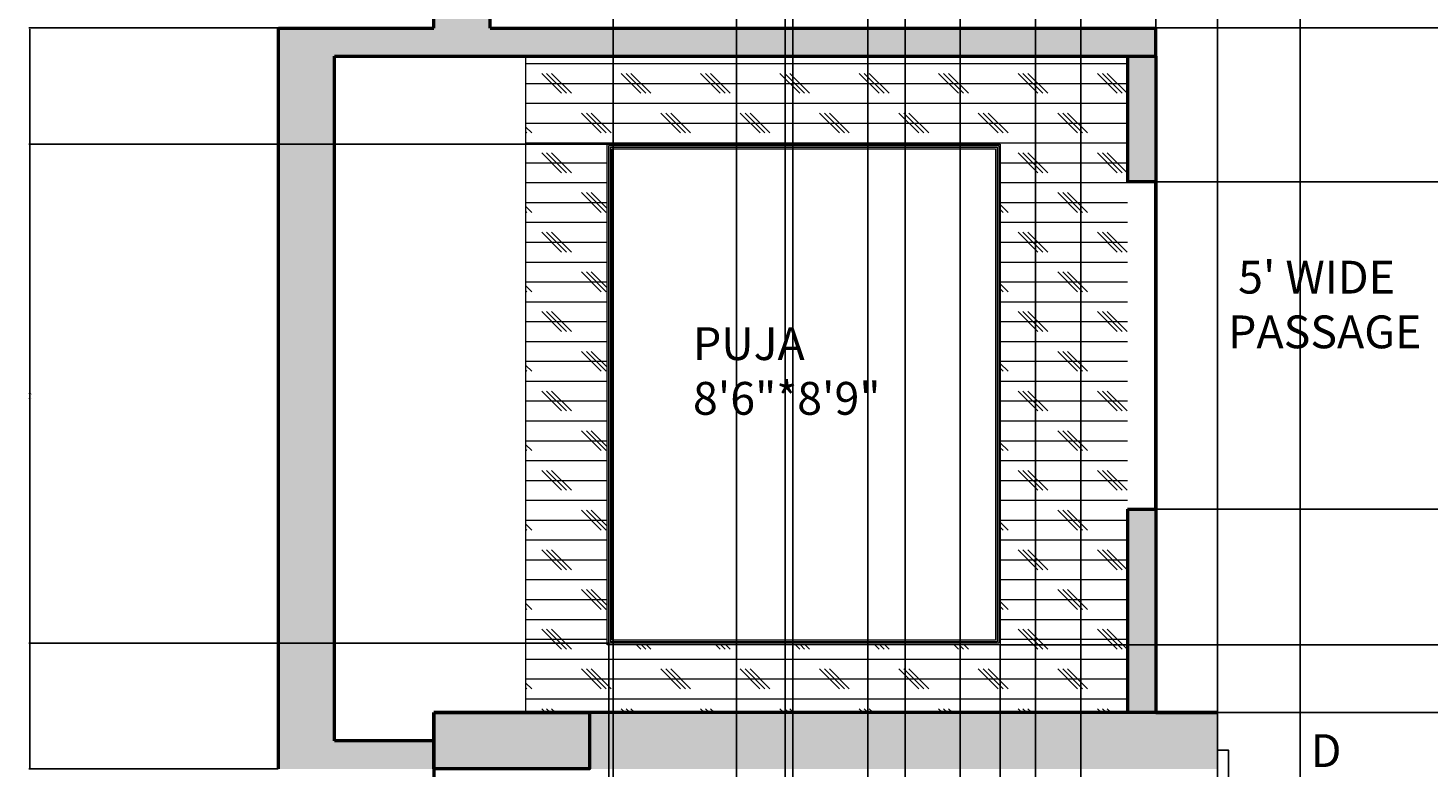
# Model space of a CAD drawing. Units: inches. Extents: x 2494 to 2908, y 1051 to 1885.
# Tile 3 of 7: x 2494 to 2718, y 1338 to 1457. Entities that reach past the tile are written whole.
import ezdxf

# ---------------------------------------------------------------- set-up
doc = ezdxf.new("R2010")
doc.units = ezdxf.units.IN
for name, color, linetype, lineweight in [('A-ANNO-DIMS', 2, 'Continuous', 18), ('A-ANNO-IDEN', 130, 'Continuous', 18), ('A-AREA-IDEN', 130, 'Continuous', 18), ('A-COLS-PATT', 200, 'Continuous', 13), ('A-FLOR-PATT', 230, 'Continuous', 13), ('A-WALL-PATT', 140, 'Continuous', 13), ('COLUMN', 200, 'Continuous', 50), ('DOOR', 50, 'Continuous', 25), ('WALL', 140, 'Continuous', 50)]:
    doc.layers.add(name, color=color, linetype=linetype, lineweight=lineweight)
doc.styles.get("Standard").update_dxf_attribs({"font": 'arial.ttf'})
doc.dimstyles.get("Standard").update_dxf_attribs({"dimtxt": 0.18, "dimasz": 0.18, "dimexe": 0.18, "dimexo": 0.0625, "dimgap": 0.09, "dimtad": 0, "dimtih": 1, "dimtoh": 1, "dimdec": 4, "dimzin": 0, "dimdsep": 46, "dimtxsty": 'Standard', "dimcen": 0.09, "dimadec": 0, "dimazin": 0, "dimtfac": 1, "dimtdec": 4, "dimtofl": 0, "dimtmove": 0, "dimatfit": 3, "dimfxl": 1, "dimtolj": 1, "dimtzin": 0, "dimarcsym": 0})

# ---------------------------------------------------------------- blocks, each defined once
blk = doc.blocks.new('*U2')
for p, q in [((0, 0), (0, -6)), ((40, 0), (40, -6))]:
    blk.add_line(p, q)
blk.add_lwpolyline([(0, 0), (0, 40), (1.75, 40), (1.75, 0)], close=True)
blk.add_arc((0, 0), 40, 0, 90)
blk = doc.blocks.new('*D28')
at = {"layer": 'A-ANNO-DIMS', "color": 0, "lineweight": -2, "transparency": 16777216}
for p, q in [((2534.34, 1456.66), (2494.47, 1456.66)), ((2494.65, 1456.48), (2494.65, 1397.59)), ((2494.65, 1338.34), (2494.65, 1397.22)), ((2534.34, 1338.16), (2494.47, 1338.16))]:
    blk.add_line(p, q, dxfattribs=at)
at = {"layer": 'A-ANNO-DIMS', "color": 0, "lineweight": 100, "transparency": 16777216}
for points in [[(2494.62, 1456.48), (2494.68, 1456.48), (2494.65, 1456.66)], [(2494.62, 1338.34), (2494.68, 1338.34), (2494.65, 1338.16)]]:
    blk.add_solid(points, dxfattribs=at)
at = {"layer": 'Defpoints', "color": 0, "lineweight": 100, "transparency": 16777216}
for p in [(2494.65, 1456.66), (2534.4, 1456.66), (2534.4, 1338.16)]:
    blk.add_point(p, dxfattribs=at)
at = {"layer": 'A-ANNO-DIMS', "color": 0, "transparency": 16777216, "insert": (2494.65, 1397.41), "char_height": 0.18, "attachment_point": 5}
blk.add_mtext('\\A1;118.5', dxfattribs=at)
blk = doc.blocks.new('*D33')
at = {"layer": 'A-ANNO-DIMS', "color": 0, "lineweight": -2, "transparency": 16777216}
for p, q in [((2697.84, 1155.22), (2697.84, 1885.09)), ((2698.02, 1884.91), (2716.38, 1884.91)), ((2735.54, 1884.91), (2717.17, 1884.91)), ((2735.72, 1155.22), (2735.72, 1885.09))]:
    blk.add_line(p, q, dxfattribs=at)
at = {"layer": 'A-ANNO-DIMS', "color": 0, "lineweight": 100, "transparency": 16777216}
for points in [[(2698.02, 1884.94), (2698.02, 1884.88), (2697.84, 1884.91)], [(2735.54, 1884.94), (2735.54, 1884.88), (2735.72, 1884.91)]]:
    blk.add_solid(points, dxfattribs=at)
at = {"layer": 'Defpoints', "color": 0, "lineweight": 100, "transparency": 16777216}
for p in [(2735.72, 1884.91), (2697.84, 1155.16), (2735.72, 1155.16)]:
    blk.add_point(p, dxfattribs=at)
at = {"layer": 'A-ANNO-DIMS', "color": 0, "transparency": 16777216, "insert": (2716.78, 1884.91), "char_height": 0.18, "attachment_point": 5}
blk.add_mtext('\\A1;37.88', dxfattribs=at)
blk = doc.blocks.new('*D34')
at = {"layer": 'A-ANNO-DIMS', "color": 0, "lineweight": -2, "transparency": 16777216}
for p, q in [((2634.69, 1155.22), (2634.69, 1885.09)), ((2634.87, 1884.91), (2665.87, 1884.91)), ((2697.66, 1884.91), (2666.66, 1884.91)), ((2697.84, 1155.22), (2697.84, 1885.09))]:
    blk.add_line(p, q, dxfattribs=at)
at = {"layer": 'A-ANNO-DIMS', "color": 0, "lineweight": 100, "transparency": 16777216}
for points in [[(2634.87, 1884.94), (2634.87, 1884.88), (2634.69, 1884.91)], [(2697.66, 1884.94), (2697.66, 1884.88), (2697.84, 1884.91)]]:
    blk.add_solid(points, dxfattribs=at)
at = {"layer": 'Defpoints', "color": 0, "lineweight": 100, "transparency": 16777216}
for p in [(2697.84, 1884.91), (2634.69, 1155.16), (2697.84, 1155.16)]:
    blk.add_point(p, dxfattribs=at)
at = {"layer": 'A-ANNO-DIMS', "color": 0, "transparency": 16777216, "insert": (2666.26, 1884.91), "char_height": 0.18, "attachment_point": 5}
blk.add_mtext('\\A1;63.15', dxfattribs=at)
blk = doc.blocks.new('*D40')
at = {"layer": 'A-ANNO-DIMS', "color": 0, "lineweight": -2, "transparency": 16777216}
for p, q in [((2615.49, 1606.59), (2615.49, 1051.41)), ((2655.49, 1606.59), (2655.49, 1051.41)), ((2615.67, 1051.59), (2635.27, 1051.59)), ((2655.31, 1051.59), (2635.71, 1051.59))]:
    blk.add_line(p, q, dxfattribs=at)
at = {"layer": 'A-ANNO-DIMS', "color": 0, "lineweight": 100, "transparency": 16777216}
for points in [[(2615.67, 1051.62), (2615.67, 1051.56), (2615.49, 1051.59)], [(2655.31, 1051.62), (2655.31, 1051.56), (2655.49, 1051.59)]]:
    blk.add_solid(points, dxfattribs=at)
at = {"layer": 'Defpoints', "color": 0, "lineweight": 100, "transparency": 16777216}
for p in [(2615.49, 1606.66), (2655.49, 1606.66), (2655.49, 1051.59)]:
    blk.add_point(p, dxfattribs=at)
at = {"layer": 'A-ANNO-DIMS', "color": 0, "transparency": 16777216, "insert": (2635.49, 1051.59), "char_height": 0.18, "attachment_point": 5}
blk.add_mtext('\\A1;40', dxfattribs=at)
blk = doc.blocks.new('*D41')
at = {"layer": 'A-ANNO-DIMS', "color": 0, "lineweight": -2, "transparency": 16777216}
for p, q in [((2684.64, 1347.22), (2684.64, 1885.09)), ((2684.82, 1884.91), (2704.42, 1884.91)), ((2724.46, 1884.91), (2704.86, 1884.91)), ((2724.64, 1347.22), (2724.64, 1885.09))]:
    blk.add_line(p, q, dxfattribs=at)
at = {"layer": 'A-ANNO-DIMS', "color": 0, "lineweight": 100, "transparency": 16777216}
for points in [[(2684.82, 1884.94), (2684.82, 1884.88), (2684.64, 1884.91)], [(2724.46, 1884.94), (2724.46, 1884.88), (2724.64, 1884.91)]]:
    blk.add_solid(points, dxfattribs=at)
at = {"layer": 'Defpoints', "color": 0, "lineweight": 100, "transparency": 16777216}
for p in [(2724.64, 1884.91), (2684.64, 1347.16), (2724.64, 1347.16)]:
    blk.add_point(p, dxfattribs=at)
at = {"layer": 'A-ANNO-DIMS', "color": 0, "transparency": 16777216, "insert": (2704.64, 1884.91), "char_height": 0.18, "attachment_point": 5}
blk.add_mtext('\\A1;40', dxfattribs=at)
blk = doc.blocks.new('*D42')
at = {"layer": 'A-ANNO-DIMS', "color": 0, "lineweight": -2, "transparency": 16777216}
for p, q in [((2674.75, 1347.22), (2674.75, 1885.09)), ((2674.93, 1884.91), (2679.3, 1884.91)), ((2684.46, 1884.91), (2680.09, 1884.91)), ((2684.64, 1347.22), (2684.64, 1885.09))]:
    blk.add_line(p, q, dxfattribs=at)
at = {"layer": 'A-ANNO-DIMS', "color": 0, "lineweight": 100, "transparency": 16777216}
for points in [[(2674.93, 1884.94), (2674.93, 1884.88), (2674.75, 1884.91)], [(2684.46, 1884.94), (2684.46, 1884.88), (2684.64, 1884.91)]]:
    blk.add_solid(points, dxfattribs=at)
at = {"layer": 'Defpoints', "color": 0, "lineweight": 100, "transparency": 16777216}
for p in [(2684.64, 1884.91), (2674.75, 1347.16), (2684.64, 1347.16)]:
    blk.add_point(p, dxfattribs=at)
at = {"layer": 'A-ANNO-DIMS', "color": 0, "transparency": 16777216, "insert": (2679.7, 1884.91), "char_height": 0.18, "attachment_point": 5}
blk.add_mtext('\\A1;9.889', dxfattribs=at)
blk = doc.blocks.new('*D46')
at = {"layer": 'A-ANNO-DIMS', "color": 0, "lineweight": -2, "transparency": 16777216}
for p, q in [((2674.81, 1432.05), (2908.18, 1432.05)), ((2908, 1431.87), (2908, 1406.05)), ((2908, 1379.87), (2908, 1405.69)), ((2674.81, 1379.69), (2908.18, 1379.69))]:
    blk.add_line(p, q, dxfattribs=at)
at = {"layer": 'A-ANNO-DIMS', "color": 0, "lineweight": 100, "transparency": 16777216}
for points in [[(2907.97, 1431.87), (2908.03, 1431.87), (2908, 1432.05)], [(2907.97, 1379.87), (2908.03, 1379.87), (2908, 1379.69)]]:
    blk.add_solid(points, dxfattribs=at)
at = {"layer": 'Defpoints', "color": 0, "lineweight": 100, "transparency": 16777216}
for p in [(2674.75, 1432.05), (2908, 1432.05), (2674.75, 1379.69)]:
    blk.add_point(p, dxfattribs=at)
at = {"layer": 'A-ANNO-DIMS', "color": 0, "transparency": 16777216, "insert": (2908, 1405.87), "char_height": 0.18, "attachment_point": 5}
blk.add_mtext('\\A1;52.36', dxfattribs=at)
blk = doc.blocks.new('*D47')
at = {"layer": 'A-ANNO-DIMS', "color": 0, "lineweight": -2, "transparency": 16777216}
for p, q in [((2674.81, 1456.66), (2908.18, 1456.66)), ((2908, 1456.48), (2908, 1444.53)), ((2908, 1432.23), (2908, 1444.17)), ((2674.81, 1432.05), (2908.18, 1432.05))]:
    blk.add_line(p, q, dxfattribs=at)
at = {"layer": 'A-ANNO-DIMS', "color": 0, "lineweight": 100, "transparency": 16777216}
for points in [[(2907.97, 1456.48), (2908.03, 1456.48), (2908, 1456.66)], [(2907.97, 1432.23), (2908.03, 1432.23), (2908, 1432.05)]]:
    blk.add_solid(points, dxfattribs=at)
at = {"layer": 'Defpoints', "color": 0, "lineweight": 100, "transparency": 16777216}
for p in [(2674.75, 1456.66), (2908, 1456.66), (2674.75, 1432.05)]:
    blk.add_point(p, dxfattribs=at)
at = {"layer": 'A-ANNO-DIMS', "color": 0, "transparency": 16777216, "insert": (2908, 1444.35), "char_height": 0.18, "attachment_point": 5}
blk.add_mtext('\\A1;24.606', dxfattribs=at)
blk = doc.blocks.new('*D49')
at = {"layer": 'A-ANNO-DIMS', "color": 0, "lineweight": -2, "transparency": 16777216}
for p, q in [((2587.26, 1358.2), (2587.26, 1051.41)), ((2649.88, 1357.95), (2649.88, 1051.41)), ((2587.44, 1051.59), (2618.17, 1051.59)), ((2649.7, 1051.59), (2618.96, 1051.59))]:
    blk.add_line(p, q, dxfattribs=at)
at = {"layer": 'A-ANNO-DIMS', "color": 0, "lineweight": 100, "transparency": 16777216}
for points in [[(2587.44, 1051.62), (2587.44, 1051.56), (2587.26, 1051.59)], [(2649.7, 1051.62), (2649.7, 1051.56), (2649.88, 1051.59)]]:
    blk.add_solid(points, dxfattribs=at)
at = {"layer": 'Defpoints', "color": 0, "lineweight": 100, "transparency": 16777216}
for p in [(2587.26, 1358.26), (2649.88, 1358.01), (2649.88, 1051.59)]:
    blk.add_point(p, dxfattribs=at)
at = {"layer": 'A-ANNO-DIMS', "color": 0, "transparency": 16777216, "insert": (2618.57, 1051.59), "char_height": 0.18, "attachment_point": 5}
blk.add_mtext('\\A1;62.62', dxfattribs=at)
blk = doc.blocks.new('*D50')
at = {"layer": 'A-ANNO-DIMS', "color": 0, "lineweight": -2, "transparency": 16777216}
for p, q in [((2586.95, 1438.09), (2494.47, 1438.09)), ((2494.65, 1437.91), (2494.65, 1398.36)), ((2494.65, 1358.44), (2494.65, 1397.99)), ((2587.2, 1358.26), (2494.47, 1358.26))]:
    blk.add_line(p, q, dxfattribs=at)
at = {"layer": 'A-ANNO-DIMS', "color": 0, "lineweight": 100, "transparency": 16777216}
for points in [[(2494.62, 1437.91), (2494.68, 1437.91), (2494.65, 1438.09)], [(2494.62, 1358.44), (2494.68, 1358.44), (2494.65, 1358.26)]]:
    blk.add_solid(points, dxfattribs=at)
at = {"layer": 'Defpoints', "color": 0, "lineweight": 100, "transparency": 16777216}
for p in [(2494.65, 1438.09), (2587.01, 1438.09), (2587.26, 1358.26)]:
    blk.add_point(p, dxfattribs=at)
at = {"layer": 'A-ANNO-DIMS', "color": 0, "transparency": 16777216, "insert": (2494.65, 1398.17), "char_height": 0.18, "attachment_point": 5}
blk.add_mtext('\\A1;79.83', dxfattribs=at)
blk = doc.blocks.new('*D51')
at = {"layer": 'A-ANNO-DIMS', "color": 0, "lineweight": -2, "transparency": 16777216}
for p, q in [((2587.26, 1358.2), (2587.26, 1051.41)), ((2559.25, 1347.09), (2559.25, 1051.41)), ((2559.43, 1051.59), (2572.88, 1051.59)), ((2587.08, 1051.59), (2573.63, 1051.59))]:
    blk.add_line(p, q, dxfattribs=at)
at = {"layer": 'A-ANNO-DIMS', "color": 0, "lineweight": 100, "transparency": 16777216}
for points in [[(2559.43, 1051.62), (2559.43, 1051.56), (2559.25, 1051.59)], [(2587.08, 1051.62), (2587.08, 1051.56), (2587.26, 1051.59)]]:
    blk.add_solid(points, dxfattribs=at)
at = {"layer": 'Defpoints', "color": 0, "lineweight": 100, "transparency": 16777216}
for p in [(2587.26, 1358.26), (2559.25, 1347.16), (2559.25, 1051.59)]:
    blk.add_point(p, dxfattribs=at)
at = {"layer": 'A-ANNO-DIMS', "color": 0, "transparency": 16777216, "insert": (2573.26, 1051.59), "char_height": 0.18, "attachment_point": 5}
blk.add_mtext('\\A1;28.01', dxfattribs=at)
blk = doc.blocks.new('*D52')
at = {"layer": 'A-ANNO-DIMS', "color": 0, "lineweight": -2, "transparency": 16777216}
for p, q in [((2649.94, 1358.01), (2908.18, 1358.01)), ((2908, 1357.83), (2908, 1352.76)), ((2908, 1347.34), (2908, 1352.4)), ((2670.31, 1347.16), (2908.18, 1347.16))]:
    blk.add_line(p, q, dxfattribs=at)
at = {"layer": 'A-ANNO-DIMS', "color": 0, "lineweight": 100, "transparency": 16777216}
for points in [[(2907.97, 1357.83), (2908.03, 1357.83), (2908, 1358.01)], [(2907.97, 1347.34), (2908.03, 1347.34), (2908, 1347.16)]]:
    blk.add_solid(points, dxfattribs=at)
at = {"layer": 'Defpoints', "color": 0, "lineweight": 100, "transparency": 16777216}
for p in [(2649.88, 1358.01), (2908, 1358.01), (2670.25, 1347.16)]:
    blk.add_point(p, dxfattribs=at)
at = {"layer": 'A-ANNO-DIMS', "color": 0, "transparency": 16777216, "insert": (2908, 1352.58), "char_height": 0.18, "attachment_point": 5}
blk.add_mtext('\\A1;10.852', dxfattribs=at)
blk = doc.blocks.new('*D60')
at = {"layer": 'A-ANNO-DIMS', "color": 0, "lineweight": -2, "transparency": 16777216}
for p, q in [((2587.96, 1514.09), (2587.96, 1051.41)), ((2607.71, 1514.09), (2607.71, 1051.41)), ((2588.14, 1051.59), (2597.45, 1051.59)), ((2607.53, 1051.59), (2598.22, 1051.59))]:
    blk.add_line(p, q, dxfattribs=at)
at = {"layer": 'A-ANNO-DIMS', "color": 0, "lineweight": 100, "transparency": 16777216}
for points in [[(2588.14, 1051.62), (2588.14, 1051.56), (2587.96, 1051.59)], [(2607.53, 1051.62), (2607.53, 1051.56), (2607.71, 1051.59)]]:
    blk.add_solid(points, dxfattribs=at)
at = {"layer": 'Defpoints', "color": 0, "lineweight": 100, "transparency": 16777216}
for p in [(2587.96, 1514.15), (2607.71, 1514.15), (2607.71, 1051.59)]:
    blk.add_point(p, dxfattribs=at)
at = {"layer": 'A-ANNO-DIMS', "color": 0, "transparency": 16777216, "insert": (2597.83, 1051.59), "char_height": 0.18, "attachment_point": 5}
blk.add_mtext('\\A1;19.76', dxfattribs=at)
blk = doc.blocks.new('*D62')
at = {"layer": 'A-ANNO-DIMS', "color": 0, "lineweight": -2, "transparency": 16777216}
for p, q in [((2616.72, 1527.95), (2616.72, 1051.41)), ((2628.68, 1527.95), (2628.68, 1051.41)), ((2616.9, 1051.59), (2622.25, 1051.59)), ((2628.5, 1051.59), (2623.16, 1051.59))]:
    blk.add_line(p, q, dxfattribs=at)
at = {"layer": 'A-ANNO-DIMS', "color": 0, "lineweight": 100, "transparency": 16777216}
for points in [[(2616.9, 1051.62), (2616.9, 1051.56), (2616.72, 1051.59)], [(2628.5, 1051.62), (2628.5, 1051.56), (2628.68, 1051.59)]]:
    blk.add_solid(points, dxfattribs=at)
at = {"layer": 'Defpoints', "color": 0, "lineweight": 100, "transparency": 16777216}
for p in [(2616.72, 1528.01), (2628.68, 1528.01), (2628.68, 1051.59)]:
    blk.add_point(p, dxfattribs=at)
at = {"layer": 'A-ANNO-DIMS', "color": 0, "transparency": 16777216, "insert": (2622.7, 1051.59), "char_height": 0.18, "attachment_point": 5}
blk.add_mtext('\\A1;11.963', dxfattribs=at)
blk = doc.blocks.new('*D65')
at = {"layer": 'A-ANNO-DIMS', "color": 0, "lineweight": -2, "transparency": 16777216}
for p, q in [((2662.76, 1694.66), (2662.76, 1051.41)), ((2643.46, 1680.73), (2643.46, 1051.41)), ((2643.64, 1051.59), (2652.66, 1051.59)), ((2662.58, 1051.59), (2653.57, 1051.59))]:
    blk.add_line(p, q, dxfattribs=at)
at = {"layer": 'A-ANNO-DIMS', "color": 0, "lineweight": 100, "transparency": 16777216}
for points in [[(2643.64, 1051.62), (2643.64, 1051.56), (2643.46, 1051.59)], [(2662.58, 1051.62), (2662.58, 1051.56), (2662.76, 1051.59)]]:
    blk.add_solid(points, dxfattribs=at)
at = {"layer": 'Defpoints', "color": 0, "lineweight": 100, "transparency": 16777216}
for p in [(2662.76, 1694.72), (2643.46, 1680.79), (2662.76, 1051.59)]:
    blk.add_point(p, dxfattribs=at)
at = {"layer": 'A-ANNO-DIMS', "color": 0, "transparency": 16777216, "insert": (2653.11, 1051.59), "char_height": 0.18, "attachment_point": 5}
blk.add_mtext('\\A1;19.305', dxfattribs=at)

msp = doc.modelspace()

# ---------------------------------------------------------------- hatches: boundary and pattern name
at = {"layer": 'A-COLS-PATT'}
h = msp.add_hatch(color=256, dxfattribs=at)
h.dxf.hatch_style = 1
h.paths.add_polyline_path([(2584.1612, 1845.1561), (2559.2517, 1845.1561), (2559.2517, 1836.1561), (2584.1612, 1836.1561)])
h.paths.add_polyline_path([(2720.7462, 1845.1561), (2695.8368, 1845.1561), (2695.8368, 1836.1561), (2720.7462, 1836.1561)])
h.paths.add_polyline_path([(2868.2517, 1845.1561), (2843.3423, 1845.1561), (2843.3423, 1836.1561), (2868.2517, 1836.1561)])
h.paths.add_polyline_path([(2568.2517, 1728.1561), (2559.2517, 1728.1561), (2559.2517, 1703.2467), (2568.2517, 1703.2467)])
h.paths.add_polyline_path([(2568.2517, 1564.0885), (2559.2517, 1564.0885), (2559.2517, 1539.1791), (2568.2517, 1539.1791)])
h.paths.add_polyline_path([(2868.2517, 1554.4528), (2859.2517, 1554.4528), (2859.2517, 1529.5434), (2868.2517, 1529.5434)])
h.paths.add_polyline_path([(2806.0841, 1611.1561), (2781.1746, 1611.1561), (2781.1746, 1602.1561), (2806.0841, 1602.1561)])
h.paths.add_polyline_path([(2868.0971, 1611.1561), (2843.1877, 1611.1561), (2843.1877, 1602.1561), (2868.0971, 1602.1561)])
h.paths.add_polyline_path([(2584.1612, 1347.1561), (2559.2517, 1347.1561), (2559.2517, 1338.1561), (2584.1612, 1338.1561)])
h.paths.add_polyline_path([(2868.2517, 1347.1561), (2843.3423, 1347.1561), (2843.3423, 1338.1561), (2868.2517, 1338.1561)])
h.paths.add_polyline_path([(2568.2517, 1180.0656), (2559.2517, 1180.0656), (2559.2517, 1155.1561), (2568.2517, 1155.1561)])
h.paths.add_polyline_path([(2584.1612, 1155.1561), (2559.2517, 1155.1561), (2559.2517, 1146.1561), (2584.1612, 1146.1561)])
h.paths.add_polyline_path([(2868.2517, 1155.1561), (2843.3423, 1155.1561), (2843.3423, 1146.1561), (2868.2517, 1146.1561)])
h.paths.add_polyline_path([(2868.2517, 1180.0656), (2859.2517, 1180.0656), (2859.2517, 1155.1561), (2868.2517, 1155.1561)])
at = {"layer": 'A-FLOR-PATT'}
h = msp.add_hatch(dxfattribs=at)
h.set_pattern_fill('CORK', color=256)
h.set_pattern_definition([(0, (0, 0), (0, 3.175), []), (135, (1.5875, -1.5875), (-6.350003, -6.350003), [4.49013, -4.49013]), (135, (2.381, -1.5875), (-6.350003, -6.350003), [4.49013, -4.49013]), (135, (3.175, -1.5875), (-6.350003, -6.350003), [4.49013, -4.49013])])
h.paths.add_polyline_path([(2670.2517, 1452.1561), (2574.0043, 1452.1561), (2574.0043, 1347.1561), (2584.1612, 1347.1561), (2670.2517, 1347.1561)])
h.paths.add_polyline_path([(2649.877, 1438.0892), (2649.877, 1358.0085), (2587.0092, 1358.0085), (2587.0092, 1438.0892)], flags=16)
h.paths.add_polyline_path([(2649.627, 1437.8392), (2649.627, 1358.2585), (2587.2592, 1358.2585), (2587.2592, 1437.8392)], flags=0)
h.paths.add_polyline_path([(2649.377, 1437.5892), (2649.377, 1358.5085), (2587.5092, 1358.5085), (2587.5092, 1437.5892)], flags=0)
h.paths.add_polyline_path([(2649.127, 1437.3392), (2649.127, 1358.7585), (2587.7592, 1358.7585), (2587.7592, 1437.3392)], flags=0)
h.paths.add_polyline_path([(2598.8437, 1391.9158), (2628.9044, 1391.9158), (2628.9044, 1411.4992), (2598.8437, 1411.4992)], flags=8)
at = {"layer": 'A-WALL-PATT'}
h = msp.add_hatch(color=256, dxfattribs=at)
h.dxf.hatch_style = 1
h.paths.add_polyline_path([(2805.2517, 1547.9123), (2796.2517, 1547.9123), (2796.2517, 1530.1561), (2859.2517, 1530.1561), (2859.2517, 1539.1561), (2805.2517, 1539.1561)])
h.paths.add_polyline_path([(2568.2517, 1606.6561), (2615.4916, 1606.6561), (2615.4916, 1611.1561), (2559.2517, 1611.1561), (2559.2517, 1564.0885), (2568.2517, 1564.0885)])
h.paths.add_polyline_path([(2568.2517, 1539.1791), (2559.2517, 1539.1791), (2559.2517, 1456.6561), (2534.4016, 1456.6561), (2534.4016, 1338.1561), (2559.2517, 1338.1561), (2559.2517, 1342.6561), (2543.4016, 1342.6561), (2543.4016, 1452.1561), (2559.2517, 1452.1561), (2568.2517, 1452.1561), (2674.7517, 1452.1561), (2674.7517, 1456.6561), (2568.2517, 1456.6561)])
h.paths.add_polyline_path([(2684.6403, 1347.1561), (2674.7517, 1347.1561), (2584.1612, 1347.1561), (2584.1612, 1338.1561), (2684.6403, 1338.1561), (2684.6403, 1341.1561)])
h.paths.add_polyline_path([(2843.3423, 1347.1561), (2832.3482, 1347.1561), (2832.3482, 1338.1485), (2843.3423, 1338.1485)])
h.paths.add_polyline_path([(2634.6908, 1155.1561), (2584.1612, 1155.1561), (2584.1612, 1146.1561), (2634.6908, 1146.1561)])
h.paths.add_polyline_path([(2783.7833, 1155.1561), (2772.2517, 1155.1561), (2772.2517, 1146.1561), (2783.7833, 1146.1561)])
h.paths.add_polyline_path([(2843.3423, 1155.1561), (2819.0012, 1155.1561), (2811.9091, 1155.1561), (2811.9091, 1146.1561), (2843.3423, 1146.1561)])
h.paths.add_polyline_path([(2868.2517, 1243.6561), (2859.2517, 1243.6561), (2859.2517, 1239.1561), (2859.2517, 1180.0656), (2868.2517, 1180.0656)])
h = msp.add_hatch(color=256, dxfattribs=at)
h.dxf.hatch_style = 1
h.paths.add_polyline_path([(2674.7517, 1379.6865), (2670.2517, 1379.6865), (2670.2517, 1347.1561), (2674.7517, 1347.1561)])
h.paths.add_polyline_path([(2674.7517, 1452.1561), (2670.2517, 1452.1561), (2670.2517, 1432.0498), (2674.7517, 1432.0498)])

# ---------------------------------------------------------------- linework, layer by layer
at = {"layer": 'A-FLOR-PATT'}
msp.add_line((2574.0043, 1347.1561), (2574.0043, 1452.1561), dxfattribs=at)
for points in [[(2587.0092, 1438.0892), (2649.877, 1438.0892), (2649.877, 1358.0085), (2587.0092, 1358.0085)], [(2587.2592, 1437.8392), (2649.627, 1437.8392), (2649.627, 1358.2585), (2587.2592, 1358.2585)], [(2587.5092, 1437.5892), (2649.377, 1437.5892), (2649.377, 1358.5085), (2587.5092, 1358.5085)], [(2587.7592, 1437.3392), (2649.127, 1437.3392), (2649.127, 1358.7585), (2587.7592, 1358.7585)]]:
    msp.add_lwpolyline(points, close=True, dxfattribs=at)
at = {"layer": 'COLUMN'}
msp.add_lwpolyline([(2559.2517, 1347.1561), (2584.1612, 1347.1561), (2584.1612, 1338.1561), (2559.2517, 1338.1561)], close=True, dxfattribs=at)
at = {"layer": 'WALL'}
for p, q in [((2559.2517, 1456.6561), (2559.2517, 1611.1561)), ((2568.2517, 1456.6561), (2568.2517, 1606.6561)), ((2534.4016, 1338.1561), (2534.4016, 1456.6561)), ((2534.4016, 1456.6561), (2559.2517, 1456.6561)), ((2568.2517, 1456.6561), (2674.7517, 1456.6561)), ((2568.2517, 1456.6561), (2674.7517, 1456.6561)), ((2674.7517, 1452.1561), (2674.7517, 1456.6561)), ((2543.4016, 1342.6561), (2543.4016, 1452.1561)), ((2543.4016, 1452.1561), (2559.2517, 1452.1561)), ((2559.2517, 1452.1561), (2568.2517, 1452.1561)), ((2568.2517, 1452.1561), (2670.2517, 1452.1561)), ((2568.2517, 1452.1561), (2674.7517, 1452.1561)), ((2670.2517, 1452.1561), (2670.2517, 1432.0498)), ((2674.7517, 1452.1561), (2674.7517, 1347.1561)), ((2670.2517, 1379.6865), (2670.2517, 1347.1561)), ((2559.2517, 1347.1561), (2559.2517, 1146.1561)), ((2684.6403, 1347.1561), (2559.2517, 1347.1561)), ((2674.7517, 1347.1561), (2684.6403, 1347.1561)), ((2559.2517, 1342.6561), (2543.4016, 1342.6561))]:
    msp.add_line(p, q, dxfattribs=at)
msp.add_lwpolyline([(2670.2517, 1379.6865), (2674.7517, 1379.6865), (2674.7517, 1432.0498), (2670.2517, 1432.0498)], dxfattribs=at)

# ---------------------------------------------------------------- block references
at = {"layer": 'DOOR', "xscale": -1, "rotation": 180}
msp.add_blockref('*U2', (2684.6403, 1341.1561), dxfattribs=at)

# ---------------------------------------------------------------- texts
at = {"layer": 'A-ANNO-IDEN', "insert": (2699.5394, 1343.7052), "char_height": 5.2482, "attachment_point": 1}
msp.add_mtext_dynamic_manual_height_columns('D', width=250.978097, gutter_width=26.2409, heights=[0], dxfattribs=at)
at = {"layer": 'A-AREA-IDEN', "char_height": 5.24818, "attachment_point": 1}
for s, insert in [(" 5' WIDE\\PPASSAGE", (2686.3269, 1419.4317)), ('PUJA\\P8\'6"*8\'9"', (2600.7214, 1408.7981))]:
    msp.add_mtext_dynamic_manual_height_columns(s, width=250.978097, gutter_width=26.2409, heights=[0], dxfattribs=dict(at, insert=insert))

# ---------------------------------------------------------------- dimensions: what is measured, and where the dimension line sits
at = {"layer": 'A-ANNO-DIMS'}
for base, p1, p2, override, picture, middle in [((2697.838, 1884.9061), (2634.6908, 1155.1561), (2697.838, 1155.1561), {"dimdec": 2, "dimlfac": 1, "dimrnd": 0, "dimzin": 0, "dimdsep": 46, "dimlunit": 2}, '*D34', (2666.2644, 1884.9061)), ((2684.6403, 1884.9061), (2674.7517, 1347.1561), (2684.6403, 1347.1561), {"dimdec": 3, "dimlfac": 1, "dimrnd": 0, "dimzin": 0, "dimdsep": 46, "dimlunit": 2}, '*D42', (2679.696, 1884.9061)), ((2724.6403, 1884.9061), (2684.6403, 1347.1561), (2724.6403, 1347.1561), {"dimdec": 0, "dimlfac": 1, "dimrnd": 0, "dimzin": 0, "dimdsep": 46, "dimlunit": 2}, '*D41', (2704.6403, 1884.9061)), ((2735.7191, 1884.9061), (2697.838, 1155.1561), (2735.7191, 1155.1561), {"dimdec": 2, "dimlfac": 1, "dimrnd": 0, "dimzin": 0, "dimdsep": 46, "dimlunit": 2}, '*D33', (2716.7785, 1884.9061)), ((2662.7647, 1051.5937), (2643.4597, 1680.7919), (2662.7647, 1694.719), {"dimdec": 3, "dimlfac": 1, "dimrnd": 0, "dimzin": 0, "dimdsep": 46, "dimlunit": 2}, '*D65', (2653.1122, 1051.5937)), ((2655.4916, 1051.5937), (2615.4916, 1606.6561), (2655.4916, 1606.6561), {"dimdec": 0, "dimlfac": 1, "dimrnd": 0, "dimzin": 0, "dimdsep": 46, "dimlunit": 2}, '*D40', (2635.4916, 1051.5937)), ((2628.6843, 1051.5937), (2616.7213, 1528.0102), (2628.6843, 1528.0102), {"dimdec": 3, "dimlfac": 1, "dimrnd": 0, "dimzin": 0, "dimdsep": 46, "dimlunit": 2}, '*D62', (2622.7028, 1051.5937)), ((2607.7136, 1051.5937), (2587.9553, 1514.1514), (2607.7136, 1514.1514), {"dimdec": 2, "dimlfac": 1, "dimrnd": 0, "dimzin": 0, "dimdsep": 46, "dimlunit": 2}, '*D60', (2597.8345, 1051.5937)), ((2559.2517, 1051.5937), (2587.2592, 1358.2585), (2559.2517, 1347.1561), {"dimdec": 2, "dimlfac": 1, "dimrnd": 0, "dimzin": 0, "dimdsep": 46, "dimlunit": 2}, '*D51', (2573.2554, 1051.5937)), ((2649.877, 1051.5937), (2587.2592, 1358.2585), (2649.877, 1358.0085), {"dimdec": 2, "dimlfac": 1, "dimrnd": 0, "dimzin": 0, "dimdsep": 46, "dimlunit": 2}, '*D49', (2618.5681, 1051.5937))]:
    dim = msp.add_linear_dim(base=base, p1=p1, p2=p2, dimstyle='Standard', override=override, dxfattribs=at)
    dim.commit()
    dim.dimension.update_dxf_attribs({"geometry": picture, "text_midpoint": middle})
for base, p1, p2, override, picture, middle in [((2494.6516, 1456.6561), (2534.4016, 1338.1561), (2534.4016, 1456.6561), {"dimdec": 1, "dimlfac": 1, "dimrnd": 0, "dimzin": 0, "dimdsep": 46, "dimlunit": 2}, '*D28', (2494.6516, 1397.4061)), ((2908.0017, 1456.6561), (2674.7517, 1432.0498), (2674.7517, 1456.6561), {"dimdec": 3, "dimlfac": 1, "dimrnd": 0, "dimzin": 0, "dimdsep": 46, "dimlunit": 2}, '*D47', (2908.0017, 1444.353)), ((2494.6516, 1438.0892), (2587.2592, 1358.2585), (2587.0092, 1438.0892), {"dimdec": 2, "dimlfac": 1, "dimrnd": 0, "dimzin": 0, "dimdsep": 46, "dimlunit": 2}, '*D50', (2494.6516, 1398.1739)), ((2908.0017, 1432.0498), (2674.7517, 1379.6865), (2674.7517, 1432.0498), {"dimdec": 2, "dimlfac": 1, "dimrnd": 0, "dimzin": 0, "dimdsep": 46, "dimlunit": 2}, '*D46', (2908.0017, 1405.8682)), ((2908.0017, 1358.0085), (2670.2517, 1347.1561), (2649.877, 1358.0085), {"dimdec": 3, "dimlfac": 1, "dimrnd": 0, "dimzin": 0, "dimdsep": 46, "dimlunit": 2}, '*D52', (2908.0017, 1352.5823))]:
    dim = msp.add_linear_dim(base=base, p1=p1, p2=p2, angle=90, dimstyle='Standard', override=override, dxfattribs=at)
    dim.commit()
    dim.dimension.update_dxf_attribs({"geometry": picture, "text_midpoint": middle})

doc.saveas('drawing.dxf')
